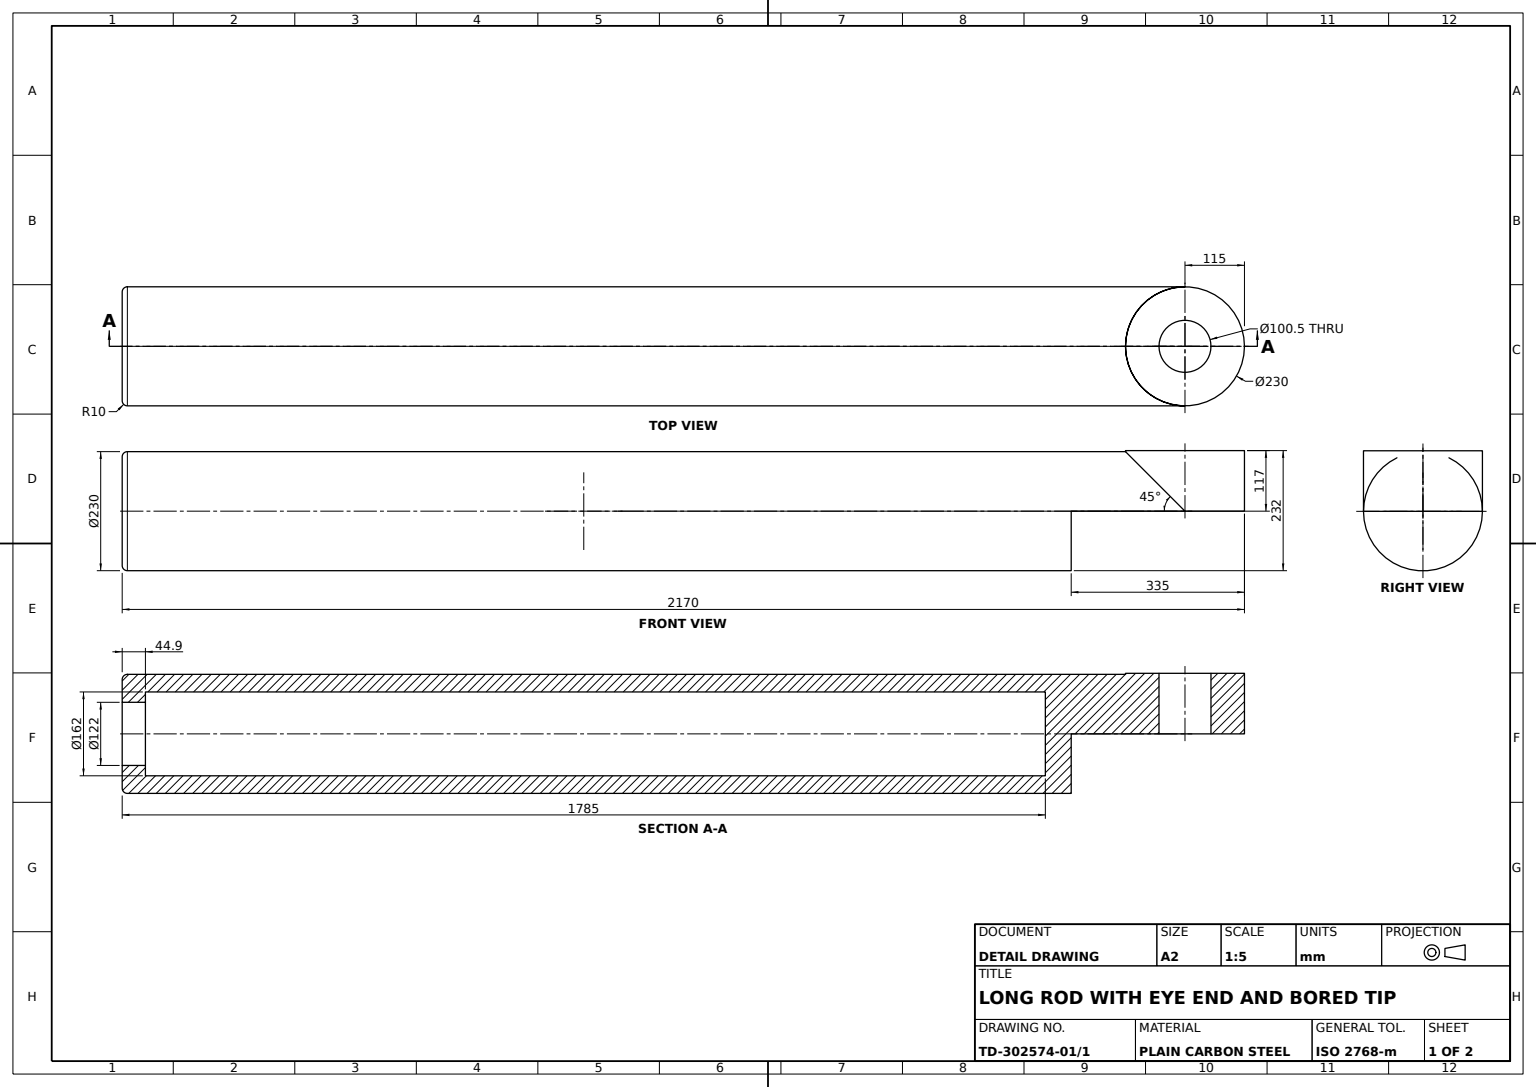
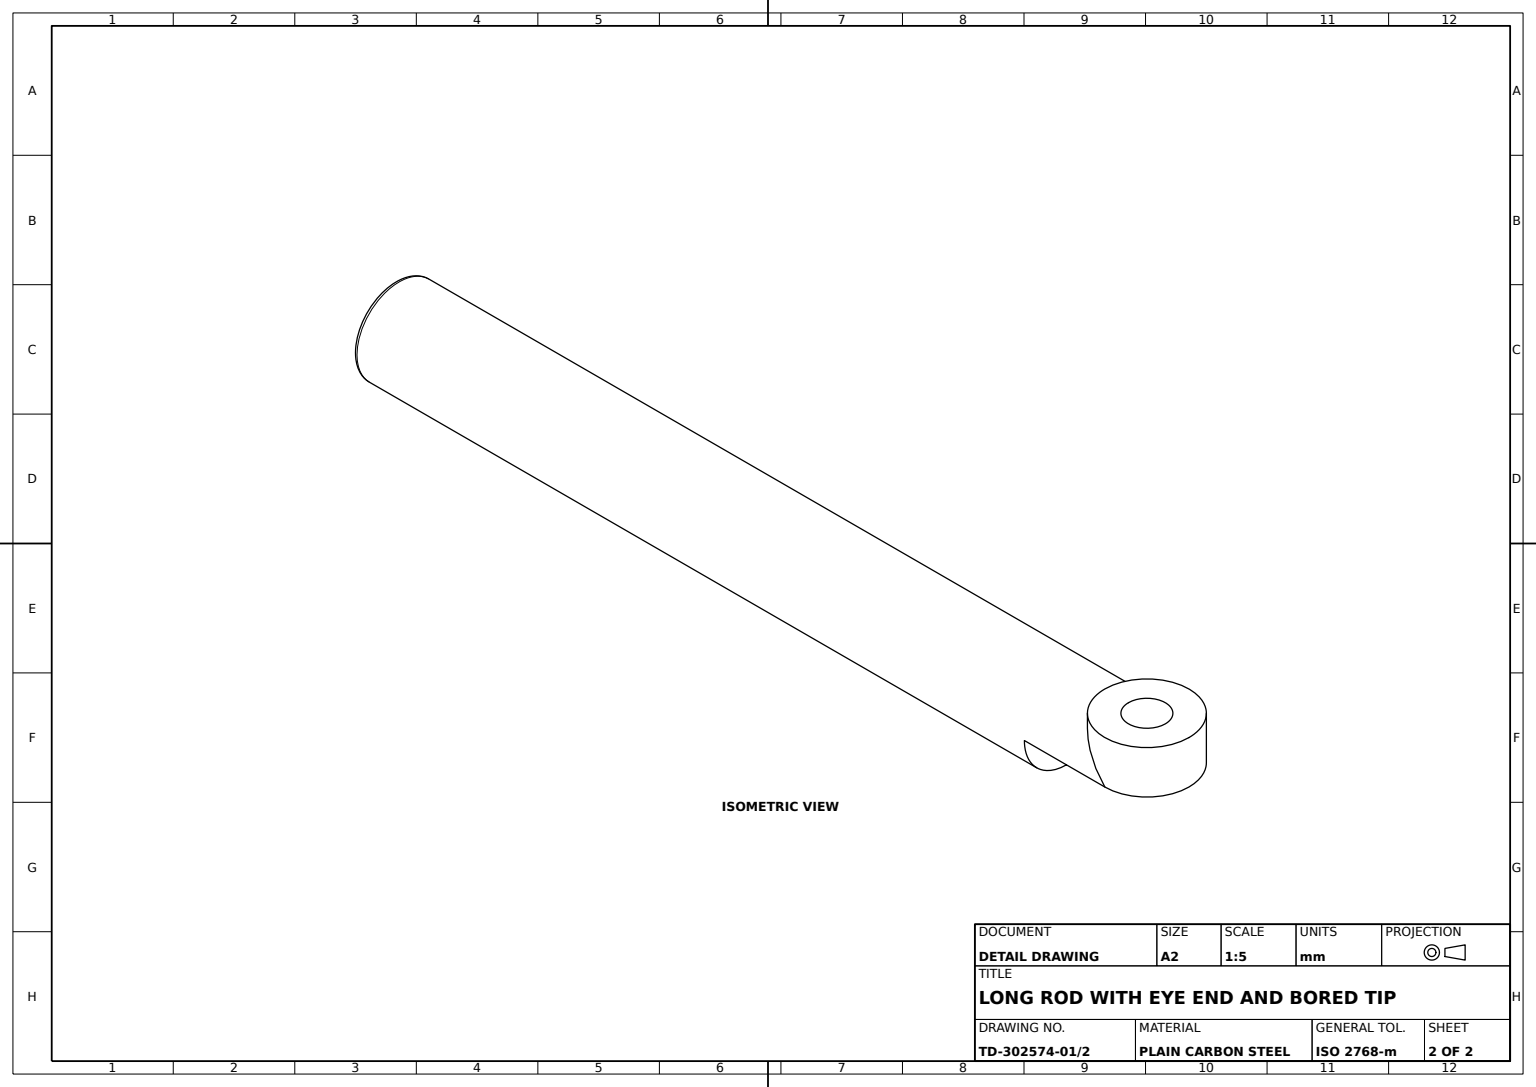
SolidWorks part; units mm, degrees
material "Plain Carbon Steel"
ref_plane "Front Plane" through (0, 0, 0) normal (0, 0, 1) x (1, 0, 0)
ref_plane "Top Plane" through (0, 0, 0) normal (0, 1, 0) x (1, 0, 0)
ref_plane "Right Plane" through (0, 0, 0) normal (1, 0, 0) x (0, 0, -1)
sketch "Barrel Profile Sketch" plane through (0, 0, 0) normal (0, 0, 1) x (1, 0, 0)
  circle A0 centre (0, 0) radius 115
  dimension "D1" = 230
extrude "Barrel Body Ø230" add sketch "Barrel Profile Sketch" along normal mid plane 2200
sketch "Eye Pin Hole Sketch" plane through (0, 0, 0) normal (0, 1, 0) x (1, 0, 0)
  circle A0 centre (0, 955) radius 50.25
  dimension "D1" = 100.5
  dimension "D2" = 955
extrude "Eye Pin Hole Ø100.5" cut sketch "Eye Pin Hole Sketch" against normal mid plane 2200
sketch "Eye Flats Sketch" plane through (0, 0, 0) normal (0, 1, 0) x (1, 0, 0)
  line L0 (115, -1100) -> (115, 1100) construction
  line L1 (-115, 1100) -> (115, 1100)
  line L2 (-115, 1100) -> (-115, 735)
  line L3 (-115, 735) -> (115, 735)
  line L4 (115, 1100) -> (115, 735)
  dimension "D1" = 365
  dimension "D2" = 230
extrude "Eye Flats Cut" cut sketch "Eye Flats Sketch" against normal blind 2200
sketch "Eye Transition Sketch" plane through (0, 0, 0) normal (0, -1, 0) x (1, 0, 0)
  line L0 (-115, -955) -> (-196.3465, -955)
  line L1 (-196.3465, -955) -> (-196.3465, -1191.8598)
  line L2 (-196.3465, -1191.8598) -> (0, -1191.8598)
  line L3 (0, -1191.8598) -> (0, -1070) construction
  line L4 (0, -1070) -> (0, -1191.8598)
  line L5 (-115, -1100) -> (-115, -735) construction
  line L6 (115, -1100) -> (-115, -1100) construction
  arc A0 (-115, -955) -> (0, -1070) centre (0, -955) ccw
  dimension "D1" = 230
  dimension "D2" = 81.3465
  dimension "D3" = 91.8598
revolve "Eye Transition Revolve Cut" cut sketch "Eye Transition Sketch" angle 360 about L3
sketch "End Bore Sketch" plane through (0, 0, 0) normal (0, 1, 0) x (1, 0, 0)
  line L0 (0, -1100) -> (0, 1148.8887) construction
  line L2 (0, -1100) -> (61, -1100)
  line L3 (61, -1100) -> (61, -1055.1029)
  line L4 (61, -1055.1029) -> (81, -1055.1029)
  line L6 (81, -1055.1029) -> (81, 685)
  line L7 (81, 685) -> (0, 685)
  line L8 (0, -1100) -> (0, 685)
  dimension "D1" = 162
  dimension "D2" = 61
  dimension "D3" = 50
  dimension "D4" = 1785
  dimension "D5" = 44.8971
revolve "End Bore Revolve Cut" cut sketch "End Bore Sketch" angle 360 about L0
sketch "Eye Boss Sketch" plane through (0, 0, 0) normal (0, -1, 0) x (1, 0, 0)
  circle A0 centre (0, -955) radius 115
  circle A1 centre (0, -955) radius 50.25 construction
  circle A2 centre (0, -955) radius 50.25
  dimension "D1" = 230
extrude "Eye Boss Extrude" add sketch "Eye Boss Sketch" against normal blind 117
fillet "Edge Fillet R10" radius 10 1 edges at (115, 0, 1100)
